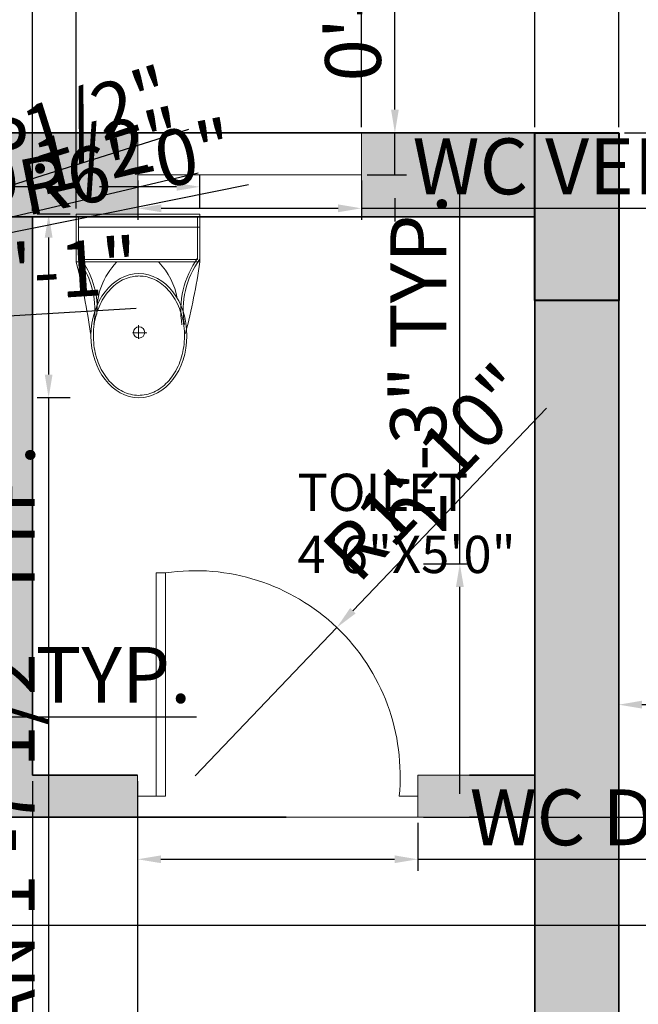
# Model space of a CAD drawing. Units: inches. Extents: x 2656 to 9931, y 1941 to 3068.
# Tile 23 of 46: x 2934 to 3000, y 2530 to 2636. Entities that reach past the tile are written whole.
import ezdxf

# ---------------------------------------------------------------- set-up
doc = ezdxf.new("R2010")
doc.units = ezdxf.units.IN
for name, color, linetype, lineweight in [('A-ANNO-DIMS', 2, 'Continuous', 18), ('A-AREA-IDEN', 7, 'Continuous', 18), ('A-COLS', 7, 'Continuous', 40), ('A-COLS-PATT', 146, 'Continuous', 13), ('A-DOOR', 3, 'Continuous', 18), ('A-FLOR-FIXT', 9, 'Continuous', 18), ('A-GLAZ', 4, 'Continuous', 18), ('A-WALL', 7, 'Continuous', 35), ('A-WALL-PATT', 251, 'Continuous', 13)]:
    doc.layers.add(name, color=color, linetype=linetype, lineweight=lineweight)
doc.styles.get("Standard").update_dxf_attribs({"font": 'arial.ttf'})
doc.dimstyles.new('ISO-25', dxfattribs={"dimtxt": 6, "dimasz": 2.5, "dimexe": 1.25, "dimexo": 0.625, "dimtad": 1, "dimdec": 0, "dimlunit": 3, "dimtxsty": 'Standard', "dimcen": 2.5, "dimadec": 0, "dimazin": 0, "dimtfac": 1, "dimtdec": 0, "dimtmove": 0, "dimatfit": 3, "dimfxl": 1, "dimarcsym": 0})

# ---------------------------------------------------------------- blocks, each defined once
blk = doc.blocks.new('*D3')
at = {"layer": 'A-ANNO-DIMS', "color": 0, "lineweight": -2, "transparency": 16777216}
for p, q in [((2998.16, 2562.82), (2998.16, 2563.44)), ((3028.16, 2562.82), (3028.16, 2563.44)), ((3000.66, 2562.19), (3025.66, 2562.19))]:
    blk.add_line(p, q, dxfattribs=at)
at = {"layer": 'A-ANNO-DIMS', "color": 0, "transparency": 16777216}
for points in [[(3000.66, 2562.61), (3000.66, 2561.77), (2998.16, 2562.19)], [(3025.66, 2562.61), (3025.66, 2561.77), (3028.16, 2562.19)]]:
    blk.add_solid(points, dxfattribs=at)
at = {"layer": 'Defpoints', "color": 0, "transparency": 16777216}
for p in [(2998.16, 2562.19), (3028.16, 2562.19), (3028.16, 2562.19)]:
    blk.add_point(p, dxfattribs=at)
at = {"layer": 'A-ANNO-DIMS', "color": 0, "transparency": 16777216, "insert": (3013.16, 2565.88), "char_height": 6, "attachment_point": 5}
blk.add_mtext('2\'6"', dxfattribs=at)
blk = doc.blocks.new('A$C31115884')
for p, q in [((283.1, 497.7), (223.4, 497.7)), ((257.5, 466.4), (257.5, 523.2)), ((0, 200), (0, 0)), ((520, 200), (0, 200)), ((10, 190), (10, 10)), ((510, 190), (10, 190)), ((510, 10), (510, 190)), ((520, 0), (520, 200)), ((510, 54.5), (0, 54.5)), ((10, 10), (510, 10)), ((0, 0), (520, 0))]:
    blk.add_line(p, q)
blk.add_circle((255.6, 496.4), 23.6)
for centre, radius, start, end in [((2777.7, -204.6), 2807, 165.4549, 171.7133), ((3237, 905), 2807, 188.2867, 194.5451), ((-294.5, 403.3), 364.7, 324.2091, 9.3499), ((-294.5, 403.3), 374.7, 324.2091, 9.3499), ((805.8, 403.3), 364.7, 170.6501, 215.7909), ((139.5, 406.2), 293.5, 315.8436, 2.6563), ((805.8, 403.3), 374.7, 179.2036, 215.7909), ((383.6, 406.2), 293.5, 190.2774, 224.1564)]:
    blk.add_arc(centre, radius, start, end)
blk.add_ellipse((256.2, 509.9), major_axis=(0, -260.7), ratio=0.772727)
blk.add_open_spline([(256.2, 259.2), (263.1, 259.2), (270, 259.7), (287.8, 262.3), (298.7, 265.1), (319.9, 273.1), (330.2, 278.4), (350.1, 291.1), (359.7, 298.7), (377.7, 315.9), (386.2, 325.5), (401.7, 346.6), (408.8, 358.1), (421.3, 382.5), (426.8, 395.5), (435.9, 422.4), (439.5, 436.4), (444.8, 465.1), (446.5, 479.7), (447.9, 509.2), (447.6, 524), (445, 553.3), (442.7, 567.8), (436.3, 596), (432.1, 609.7), (421.9, 636), (416, 648.6), (402.5, 672.1), (395, 683), (378.6, 703), (369.8, 712.1), (351.1, 728), (341.3, 734.8), (320.9, 746.2), (310.4, 750.7), (288.9, 757.3), (278, 759.4), (256, 761), (245, 760.6), (223.1, 757.2), (212.3, 754.3), (191.1, 746.1), (180.8, 740.7), (160.9, 727.8), (151.4, 720.1), (133.5, 702.7), (125.1, 693), (109.6, 671.7), (102.6, 660.2), (90.2, 635.7), (84.9, 622.7), (76, 595.6), (72.4, 581.6), (67.2, 552.9), (65.6, 538.2), (64.4, 508.8), (64.8, 494), (67.5, 464.7), (69.9, 450.2), (76.6, 422), (80.8, 408.3), (91.1, 382.2), (97.2, 369.7), (110.8, 346.3), (118.4, 335.4), (134.8, 315.6), (143.7, 306.7), (162.4, 290.9), (172.3, 284.2), (192.8, 273), (203.3, 268.6), (224.8, 262.2), (235.8, 260.2), (249.9, 259.3), (253, 259.2), (256.2, 259.2)], degree=3, knots=[0, 0, 0, 0, 0.110105, 0.110105, 0.285049, 0.285049, 0.459994, 0.459994, 0.634938, 0.634938, 0.809882, 0.809882, 0.984827, 0.984827, 1.159771, 1.159771, 1.334715, 1.334715, 1.50966, 1.50966, 1.684604, 1.684604, 1.859549, 1.859549, 2.034493, 2.034493, 2.209437, 2.209437, 2.384382, 2.384382, 2.559326, 2.559326, 2.73427, 2.73427, 2.909215, 2.909215, 3.084159, 3.084159, 3.259103, 3.259103, 3.434048, 3.434048, 3.608992, 3.608992, 3.783936, 3.783936, 3.958881, 3.958881, 4.133825, 4.133825, 4.30877, 4.30877, 4.483714, 4.483714, 4.658658, 4.658658, 4.833603, 4.833603, 5.008547, 5.008547, 5.183491, 5.183491, 5.358436, 5.358436, 5.53338, 5.53338, 5.708324, 5.708324, 5.883269, 5.883269, 6.058213, 6.058213, 6.233158, 6.233158, 6.283185, 6.283185, 6.283185, 6.283185])
blk = doc.blocks.new('DOOR-WC-FRONT')
for p, q in [((1.97, 2.25), (1.97, 26.25)), ((1.97, 26.25), (2.97, 26.25)), ((2.97, 26.25), (2.97, 2.25)), ((-0.03, 2.25), (1.97, 2.25)), ((2.97, 2.25), (1.97, 2.25)), ((30.07, 2.25), (28.07, 2.25)), ((-0.03, 0), (30.07, 0))]:
    blk.add_line(p, q)
blk.add_arc((6.14, 4.44), 22.04, 354.3038, 98.2673)
blk = doc.blocks.new('WIN-VENT-24IN-B')
for p, q in [((24.01, 0), (24.01, 4.5)), ((0.01, 0), (0.01, 0)), ((0.01, 0), (24.01, 0))]:
    blk.add_line(p, q)
blk = doc.blocks.new('*D29')
at = {"layer": 'A-ANNO-DIMS', "color": 0, "lineweight": -2, "transparency": 16777216}
for p, q in [((2939.24, 2614.86), (2935.66, 2614.86)), ((2936.91, 2612.36), (2936.91, 2597.65)), ((2939.24, 2595.15), (2935.66, 2595.15)), ((2936.91, 2595.15), (2936.91, 2504.75))]:
    blk.add_line(p, q, dxfattribs=at)
at = {"layer": 'A-ANNO-DIMS', "color": 0, "transparency": 16777216}
for points in [[(2936.49, 2612.36), (2937.33, 2612.36), (2936.91, 2614.86)], [(2936.49, 2597.65), (2937.33, 2597.65), (2936.91, 2595.15)]]:
    blk.add_solid(points, dxfattribs=at)
at = {"layer": 'Defpoints', "color": 0, "transparency": 16777216}
for p in [(2939.87, 2614.86), (2936.91, 2595.15), (2939.87, 2595.15)]:
    blk.add_point(p, dxfattribs=at)
at = {"layer": 'A-ANNO-DIMS', "color": 0, "transparency": 16777216, "insert": (2933.18, 2548.7), "char_height": 6, "attachment_point": 5, "rotation": 90}
blk.add_mtext('WC PAN 1\'-7 1/2" TYP.', dxfattribs=at)
blk = doc.blocks.new('*D30')
at = {"layer": 'A-ANNO-DIMS', "color": 0, "lineweight": -2, "transparency": 16777216}
for p, q in [((2939.87, 2615.48), (2939.87, 2619.06)), ((2953.16, 2615.48), (2953.16, 2619.06)), ((2939.87, 2617.81), (2886.13, 2617.81)), ((2950.66, 2617.81), (2942.37, 2617.81))]:
    blk.add_line(p, q, dxfattribs=at)
at = {"layer": 'A-ANNO-DIMS', "color": 0, "transparency": 16777216}
for points in [[(2942.37, 2618.23), (2942.37, 2617.39), (2939.87, 2617.81)], [(2950.66, 2618.23), (2950.66, 2617.39), (2953.16, 2617.81)]]:
    blk.add_solid(points, dxfattribs=at)
at = {"layer": 'Defpoints', "color": 0, "transparency": 16777216}
for p in [(2939.87, 2617.81), (2939.87, 2614.86), (2953.16, 2614.86)]:
    blk.add_point(p, dxfattribs=at)
at = {"layer": 'A-ANNO-DIMS', "color": 0, "transparency": 16777216, "insert": (2911.75, 2621.54), "char_height": 6, "attachment_point": 5}
blk.add_mtext('1\'-1 1/2" TYP.', dxfattribs=at)
blk = doc.blocks.new('*D34')
at = {"layer": 'A-ANNO-DIMS', "color": 0, "lineweight": -2, "transparency": 16777216}
for p, q in [((2872.16, 2564.71), (2872.16, 2559.64)), ((2898.41, 2564.71), (2898.41, 2559.64)), ((2874.66, 2560.89), (2895.91, 2560.89)), ((2898.41, 2560.89), (2952.81, 2560.89))]:
    blk.add_line(p, q, dxfattribs=at)
at = {"layer": 'A-ANNO-DIMS', "color": 0, "transparency": 16777216}
for points in [[(2874.66, 2561.3), (2874.66, 2560.47), (2872.16, 2560.89)], [(2895.91, 2561.3), (2895.91, 2560.47), (2898.41, 2560.89)]]:
    blk.add_solid(points, dxfattribs=at)
at = {"layer": 'Defpoints', "color": 0, "transparency": 16777216}
for p in [(2872.16, 2565.34), (2898.41, 2565.34), (2898.41, 2560.89)]:
    blk.add_point(p, dxfattribs=at)
at = {"layer": 'A-ANNO-DIMS', "color": 0, "transparency": 16777216, "insert": (2926.86, 2564.61), "char_height": 6, "attachment_point": 5}
blk.add_mtext('2\'-2 1/2" TYP.', dxfattribs=at)
blk = doc.blocks.new('*D35')
at = {"layer": 'A-ANNO-DIMS', "color": 0, "lineweight": -2, "transparency": 16777216}
for p, q in [((2946.47, 2549.48), (2946.47, 2544.33)), ((2976.57, 2549.48), (2976.57, 2544.33)), ((2948.97, 2545.58), (2974.07, 2545.58)), ((2976.57, 2545.58), (3060.91, 2545.58))]:
    blk.add_line(p, q, dxfattribs=at)
at = {"layer": 'A-ANNO-DIMS', "color": 0, "transparency": 16777216}
for points in [[(2948.97, 2546), (2948.97, 2545.17), (2946.47, 2545.58)], [(2974.07, 2546), (2974.07, 2545.17), (2976.57, 2545.58)]]:
    blk.add_solid(points, dxfattribs=at)
at = {"layer": 'Defpoints', "color": 0, "transparency": 16777216}
for p in [(2946.47, 2550.1), (2976.57, 2550.1), (2976.57, 2545.58)]:
    blk.add_point(p, dxfattribs=at)
at = {"layer": 'A-ANNO-DIMS', "color": 0, "transparency": 16777216, "insert": (3019.99, 2549.31), "char_height": 6, "attachment_point": 5}
blk.add_mtext('WC DOOR 2\'-6" TYP.', dxfattribs=at)
blk = doc.blocks.new('*D36')
at = {"layer": 'A-ANNO-DIMS', "color": 0, "lineweight": -2, "transparency": 16777216}
for p, q in [((2981.09, 2577.33), (2981.09, 2617.75)), ((2977.2, 2577.33), (2982.34, 2577.33)), ((2981.09, 2552.6), (2981.09, 2574.83)), ((2977.2, 2550.1), (2982.34, 2550.1))]:
    blk.add_line(p, q, dxfattribs=at)
at = {"layer": 'A-ANNO-DIMS', "color": 0, "transparency": 16777216}
for points in [[(2980.67, 2574.83), (2981.51, 2574.83), (2981.09, 2577.33)], [(2980.67, 2552.6), (2981.51, 2552.6), (2981.09, 2550.1)]]:
    blk.add_solid(points, dxfattribs=at)
at = {"layer": 'Defpoints', "color": 0, "transparency": 16777216}
for p in [(2976.57, 2577.33), (2981.09, 2577.33), (2976.57, 2550.1)]:
    blk.add_point(p, dxfattribs=at)
at = {"layer": 'A-ANNO-DIMS', "color": 0, "transparency": 16777216, "insert": (2977.4, 2598.79), "char_height": 6, "attachment_point": 5, "rotation": 90}
blk.add_mtext('2\'-3" TYP.', dxfattribs=at)
blk = doc.blocks.new('*D45')
at = {"layer": 'A-ANNO-DIMS', "color": 0, "lineweight": -2, "transparency": 16777216}
for p, q in [((2946.51, 2618.48), (2946.51, 2614.25)), ((2970.51, 2618.48), (2970.51, 2614.25)), ((2949.01, 2615.5), (2968.01, 2615.5)), ((2970.51, 2615.5), (3052.06, 2615.5))]:
    blk.add_line(p, q, dxfattribs=at)
at = {"layer": 'A-ANNO-DIMS', "color": 0, "transparency": 16777216}
for points in [[(2949.01, 2615.92), (2949.01, 2615.08), (2946.51, 2615.5)], [(2968.01, 2615.92), (2968.01, 2615.08), (2970.51, 2615.5)]]:
    blk.add_solid(points, dxfattribs=at)
at = {"layer": 'Defpoints', "color": 0, "transparency": 16777216}
for p in [(2946.51, 2619.1), (2970.51, 2619.1), (2970.51, 2615.5)]:
    blk.add_point(p, dxfattribs=at)
at = {"layer": 'A-ANNO-DIMS', "color": 0, "transparency": 16777216, "insert": (3012.54, 2619.23), "char_height": 6, "attachment_point": 5}
blk.add_mtext('WC VENT 2\'-0" TYP.', dxfattribs=at)
blk = doc.blocks.new('*D46')
at = {"layer": 'A-ANNO-DIMS', "color": 0, "lineweight": -2, "transparency": 16777216}
for p, q in [((2974.11, 2626.1), (2974.11, 2680.4)), ((2971.14, 2623.6), (2975.36, 2623.6)), ((2974.11, 2619.1), (2974.11, 2623.6)), ((2971.14, 2619.1), (2975.36, 2619.1)), ((2974.11, 2616.6), (2974.11, 2614.1))]:
    blk.add_line(p, q, dxfattribs=at)
at = {"layer": 'A-ANNO-DIMS', "color": 0, "transparency": 16777216}
for points in [[(2973.7, 2626.1), (2974.53, 2626.1), (2974.11, 2623.6)], [(2973.7, 2616.6), (2974.53, 2616.6), (2974.11, 2619.1)]]:
    blk.add_solid(points, dxfattribs=at)
at = {"layer": 'Defpoints', "color": 0, "transparency": 16777216}
for p in [(2970.51, 2623.6), (2974.11, 2623.6), (2970.51, 2619.1)]:
    blk.add_point(p, dxfattribs=at)
at = {"layer": 'A-ANNO-DIMS', "color": 0, "transparency": 16777216, "insert": (2970.39, 2654.5), "char_height": 6, "attachment_point": 5, "rotation": 90}
blk.add_mtext('0\'-4 1/2" TYP.', dxfattribs=at)
blk = doc.blocks.new('*D99')
at = {"layer": 'A-ANNO-DIMS', "color": 0, "lineweight": -2, "transparency": 16777216}
for p, q in [((2970.51, 2624.23), (2970.51, 2674.45)), ((2989.16, 2624.23), (2989.16, 2674.45)), ((2973.01, 2673.2), (2986.66, 2673.2)), ((2989.16, 2673.2), (3022.27, 2673.2))]:
    blk.add_line(p, q, dxfattribs=at)
at = {"layer": 'A-ANNO-DIMS', "color": 0, "transparency": 16777216}
for points in [[(2973.01, 2673.62), (2973.01, 2672.78), (2970.51, 2673.2)], [(2986.66, 2673.62), (2986.66, 2672.78), (2989.16, 2673.2)]]:
    blk.add_solid(points, dxfattribs=at)
at = {"layer": 'Defpoints', "color": 0, "transparency": 16777216}
for p in [(2989.16, 2673.2), (2970.51, 2623.6), (2989.16, 2623.6)]:
    blk.add_point(p, dxfattribs=at)
at = {"layer": 'A-ANNO-DIMS', "color": 0, "transparency": 16777216, "insert": (3006.97, 2676.93), "char_height": 6, "attachment_point": 5}
blk.add_mtext('1\'-6 1/2"', dxfattribs=at)
blk = doc.blocks.new('*D101')
at = {"layer": 'A-ANNO-DIMS', "color": 0, "lineweight": -2, "transparency": 16777216}
for p, q in [((2935.16, 2553.98), (2935.16, 2009.27)), ((2946.47, 2553.98), (2946.47, 2009.27)), ((2937.66, 2010.52), (2943.97, 2010.52)), ((2946.47, 2010.52), (2984.81, 2010.52))]:
    blk.add_line(p, q, dxfattribs=at)
at = {"layer": 'A-ANNO-DIMS', "color": 0, "transparency": 16777216}
for points in [[(2937.66, 2010.94), (2937.66, 2010.11), (2935.16, 2010.52)], [(2943.97, 2010.94), (2943.97, 2010.11), (2946.47, 2010.52)]]:
    blk.add_solid(points, dxfattribs=at)
at = {"layer": 'Defpoints', "color": 0, "transparency": 16777216}
for p in [(2935.16, 2554.6), (2946.47, 2554.6), (2946.47, 2010.52)]:
    blk.add_point(p, dxfattribs=at)
at = {"layer": 'A-ANNO-DIMS', "color": 0, "transparency": 16777216, "insert": (2966.89, 2014.25), "char_height": 6, "attachment_point": 5}
blk.add_mtext('0\'-11 1/2"', dxfattribs=at)
blk = doc.blocks.new('*D102')
at = {"layer": 'A-ANNO-DIMS', "color": 0, "lineweight": -2, "transparency": 16777216}
for p, q in [((2998.16, 2604.98), (2998.16, 2009.27)), ((2872.16, 2564.71), (2872.16, 2009.27)), ((2874.66, 2010.52), (2995.66, 2010.52))]:
    blk.add_line(p, q, dxfattribs=at)
at = {"layer": 'A-ANNO-DIMS', "color": 0, "transparency": 16777216}
for points in [[(2874.66, 2010.94), (2874.66, 2010.11), (2872.16, 2010.52)], [(2995.66, 2010.94), (2995.66, 2010.11), (2998.16, 2010.52)]]:
    blk.add_solid(points, dxfattribs=at)
at = {"layer": 'Defpoints', "color": 0, "transparency": 16777216}
for p in [(2998.16, 2605.6), (2872.16, 2565.34), (2998.16, 2010.52)]:
    blk.add_point(p, dxfattribs=at)
at = {"layer": 'A-ANNO-DIMS', "color": 0, "transparency": 16777216, "insert": (2935.16, 2014.21), "char_height": 6, "attachment_point": 5}
blk.add_mtext('10\'-6"', dxfattribs=at)
blk = doc.blocks.new('*D103')
at = {"layer": 'A-ANNO-DIMS', "color": 0, "lineweight": -2, "transparency": 16777216}
for p, q in [((2998.78, 2623.6), (3061.01, 2623.6)), ((3059.76, 2552.6), (3059.76, 2621.1)), ((2989.78, 2550.1), (3061.01, 2550.1))]:
    blk.add_line(p, q, dxfattribs=at)
at = {"layer": 'A-ANNO-DIMS', "color": 0, "transparency": 16777216}
for points in [[(3059.34, 2621.1), (3060.17, 2621.1), (3059.76, 2623.6)], [(3059.34, 2552.6), (3060.17, 2552.6), (3059.76, 2550.1)]]:
    blk.add_solid(points, dxfattribs=at)
at = {"layer": 'Defpoints', "color": 0, "transparency": 16777216}
for p in [(2998.16, 2623.6), (3059.76, 2623.6), (2989.16, 2550.1)]:
    blk.add_point(p, dxfattribs=at)
at = {"layer": 'A-ANNO-DIMS', "color": 0, "transparency": 16777216, "insert": (3056.03, 2586.85), "char_height": 6, "attachment_point": 5, "rotation": 90}
blk.add_mtext('6\'-1 1/2"', dxfattribs=at)
blk = doc.blocks.new('*D130')
at = {"layer": 'A-ANNO-DIMS', "color": 0, "lineweight": -2, "transparency": 16777216}
for p, q in [((2877.28, 2538.52), (3061.01, 2538.52)), ((3059.76, 2536.02), (3059.76, 2525.32)), ((2902.17, 2522.82), (3061.01, 2522.82)), ((3059.76, 2522.82), (3059.76, 2489.7))]:
    blk.add_line(p, q, dxfattribs=at)
at = {"layer": 'A-ANNO-DIMS', "color": 0, "transparency": 16777216}
for points in [[(3059.34, 2536.02), (3060.17, 2536.02), (3059.76, 2538.52)], [(3059.34, 2525.32), (3060.17, 2525.32), (3059.76, 2522.82)]]:
    blk.add_solid(points, dxfattribs=at)
at = {"layer": 'Defpoints', "color": 0, "transparency": 16777216}
for p in [(2876.66, 2538.52), (2901.54, 2522.82), (3059.76, 2522.82)]:
    blk.add_point(p, dxfattribs=at)
at = {"layer": 'A-ANNO-DIMS', "color": 0, "transparency": 16777216, "insert": (3056.03, 2505.01), "char_height": 6, "attachment_point": 5, "rotation": 90}
blk.add_mtext('1\'-3 1/2"', dxfattribs=at)
blk = doc.blocks.new('*D174')
at = {"layer": 'A-ANNO-DIMS', "color": 0, "lineweight": -2, "transparency": 16777216}
for p, q in [((2743.16, 2624.23), (2743.16, 2674.45)), ((2998.16, 2624.23), (2998.16, 2674.45)), ((2745.66, 2673.2), (2995.66, 2673.2))]:
    blk.add_line(p, q, dxfattribs=at)
at = {"layer": 'A-ANNO-DIMS', "color": 0, "transparency": 16777216}
for points in [[(2745.66, 2673.62), (2745.66, 2672.78), (2743.16, 2673.2)], [(2995.66, 2673.62), (2995.66, 2672.78), (2998.16, 2673.2)]]:
    blk.add_solid(points, dxfattribs=at)
at = {"layer": 'Defpoints', "color": 0, "transparency": 16777216}
for p in [(2998.16, 2673.2), (2743.16, 2623.6), (2998.16, 2623.6)]:
    blk.add_point(p, dxfattribs=at)
at = {"layer": 'A-ANNO-DIMS', "color": 0, "transparency": 16777216, "insert": (2870.66, 2676.89), "char_height": 6, "attachment_point": 5}
blk.add_mtext('21\'-3"', dxfattribs=at)
blk = doc.blocks.new('*D177')
at = {"layer": 'A-ANNO-DIMS', "color": 0, "lineweight": -2, "transparency": 16777216}
for p, q in [((2935.16, 2615.23), (2935.16, 2674.45)), ((2939.87, 2615.48), (2939.87, 2674.45)), ((2932.66, 2673.2), (2930.16, 2673.2)), ((2935.16, 2673.2), (2939.87, 2673.2)), ((2942.37, 2673.2), (2976.05, 2673.2))]:
    blk.add_line(p, q, dxfattribs=at)
at = {"layer": 'A-ANNO-DIMS', "color": 0, "transparency": 16777216}
for points in [[(2932.66, 2673.62), (2932.66, 2672.78), (2935.16, 2673.2)], [(2942.37, 2673.62), (2942.37, 2672.78), (2939.87, 2673.2)]]:
    blk.add_solid(points, dxfattribs=at)
at = {"layer": 'Defpoints', "color": 0, "transparency": 16777216}
for p in [(2939.87, 2673.2), (2935.16, 2614.6), (2939.87, 2614.86)]:
    blk.add_point(p, dxfattribs=at)
at = {"layer": 'A-ANNO-DIMS', "color": 0, "transparency": 16777216, "insert": (2960.46, 2676.93), "char_height": 6, "attachment_point": 5}
blk.add_mtext('0\'-4 1/2"', dxfattribs=at)
blk = doc.blocks.new('*D187')
at = {"layer": 'A-ANNO-DIMS', "color": 0, "lineweight": -2, "transparency": 16777216}
for p, q in [((2990.41, 2594.03), (2969.6, 2572.28)), ((2952.64, 2554.54), (2967.87, 2570.47))]:
    blk.add_line(p, q, dxfattribs=at)
at = {"layer": 'A-ANNO-DIMS', "color": 0, "transparency": 16777216}
blk.add_solid([(2969.3, 2572.56), (2969.9, 2571.99), (2967.87, 2570.47)], dxfattribs=at)
at = {"layer": 'Defpoints', "color": 0, "transparency": 16777216}
for p in [(2967.87, 2570.47), (2952.64, 2554.54)]:
    blk.add_point(p, dxfattribs=at)
at = {"layer": 'A-ANNO-DIMS', "color": 0, "transparency": 16777216, "insert": (2978.2, 2586.61), "char_height": 6, "attachment_point": 5, "rotation": 46.2844}
blk.add_mtext('R1\'-10"', dxfattribs=at)
blk = doc.blocks.new('*D189')
at = {"layer": 'A-ANNO-DIMS', "color": 0, "lineweight": -2, "transparency": 16777216}
for p, q in [((2958.39, 2618.02), (2900.95, 2606.42)), ((2828.14, 2591.72), (2898.5, 2605.92))]:
    blk.add_line(p, q, dxfattribs=at)
at = {"layer": 'A-ANNO-DIMS', "color": 0, "transparency": 16777216}
blk.add_solid([(2900.86, 2606.83), (2901.03, 2606.01), (2898.5, 2605.92)], dxfattribs=at)
at = {"layer": 'Defpoints', "color": 0, "transparency": 16777216}
for p in [(2898.5, 2605.92), (2828.14, 2591.72)]:
    blk.add_point(p, dxfattribs=at)
at = {"layer": 'A-ANNO-DIMS', "color": 0, "transparency": 16777216, "insert": (2939.98, 2618.06), "char_height": 6, "attachment_point": 5, "rotation": 11.4157}
blk.add_mtext('4X R6\'-0"', dxfattribs=at)
blk = doc.blocks.new('*D190')
at = {"layer": 'A-ANNO-DIMS', "color": 0, "lineweight": -2, "transparency": 16777216}
for p, q in [((2951.95, 2623.98), (2901.83, 2608.18)), ((2890.31, 2604.54), (2899.44, 2607.42))]:
    blk.add_line(p, q, dxfattribs=at)
at = {"layer": 'A-ANNO-DIMS', "color": 0, "transparency": 16777216}
blk.add_solid([(2901.7, 2608.57), (2901.95, 2607.78), (2899.44, 2607.42)], dxfattribs=at)
at = {"layer": 'Defpoints', "color": 0, "transparency": 16777216}
for p in [(2899.44, 2607.42), (2890.31, 2604.54)]:
    blk.add_point(p, dxfattribs=at)
at = {"layer": 'A-ANNO-DIMS', "color": 0, "transparency": 16777216, "insert": (2926.96, 2620.01), "char_height": 6, "attachment_point": 5, "rotation": 17.4987}
blk.add_mtext('4X R0\'-9 1/2"', dxfattribs=at)
blk = doc.blocks.new('*D191')
at = {"layer": 'A-ANNO-DIMS', "color": 0, "lineweight": -2, "transparency": 16777216}
for p, q in [((2952.98, 2619.27), (2901.82, 2607.25)), ((2890.31, 2604.54), (2899.39, 2606.68))]:
    blk.add_line(p, q, dxfattribs=at)
at = {"layer": 'A-ANNO-DIMS', "color": 0, "transparency": 16777216}
blk.add_solid([(2901.72, 2607.65), (2901.91, 2606.84), (2899.39, 2606.68)], dxfattribs=at)
at = {"layer": 'Defpoints', "color": 0, "transparency": 16777216}
for p in [(2899.39, 2606.68), (2890.31, 2604.54)]:
    blk.add_point(p, dxfattribs=at)
at = {"layer": 'A-ANNO-DIMS', "color": 0, "transparency": 16777216, "insert": (2927.76, 2617.17), "char_height": 6, "attachment_point": 5, "rotation": 13.2221}
blk.add_mtext('4X R0\'-9 1/2"', dxfattribs=at)
blk = doc.blocks.new('*D193')
at = {"layer": 'A-ANNO-DIMS', "color": 0, "lineweight": -2, "transparency": 16777216}
for p, q in [((2946.3, 2604.75), (2907.47, 2602.35)), ((2901.28, 2601.97), (2898.78, 2601.82)), ((2903.77, 2602.12), (2904.98, 2602.2))]:
    blk.add_line(p, q, dxfattribs=at)
at = {"layer": 'A-ANNO-DIMS', "color": 0, "transparency": 16777216}
for points in [[(2907.45, 2602.77), (2907.5, 2601.94), (2904.98, 2602.2)], [(2901.25, 2602.39), (2901.3, 2601.55), (2903.77, 2602.12)]]:
    blk.add_solid(points, dxfattribs=at)
at = {"layer": 'Defpoints', "color": 0, "transparency": 16777216}
for p in [(2903.77, 2602.12), (2904.98, 2602.2)]:
    blk.add_point(p, dxfattribs=at)
at = {"layer": 'A-ANNO-DIMS', "color": 0, "transparency": 16777216, "insert": (2927.9, 2607.48), "char_height": 6, "attachment_point": 5, "rotation": 3.5337}
blk.add_mtext('2X ∅0\'-1"', dxfattribs=at)

msp = doc.modelspace()

# ---------------------------------------------------------------- hatches: boundary and pattern name
at = {"layer": 'A-COLS-PATT'}
h = msp.add_hatch(color=256, dxfattribs=at)
h.dxf.hatch_style = 1
h.paths.add_polyline_path([(2752.16, 2623.6), (2743.16, 2623.6), (2743.16, 2605.6), (2752.16, 2605.6)])
h.paths.add_polyline_path([(2876.66, 2623.6), (2858.66, 2623.6), (2858.66, 2614.6), (2876.66, 2614.6)])
h.paths.add_polyline_path([(2998.16, 2623.6), (2989.16, 2623.6), (2989.16, 2614.6), (2989.16, 2605.6), (2998.16, 2605.6)])
h.paths.add_polyline_path([(2998.16, 2444.1), (2989.16, 2444.1), (2989.16, 2426.1), (2998.16, 2426.1)])
h.paths.add_polyline_path([(2876.66, 2444.1), (2867.66, 2444.1), (2867.66, 2426.1), (2876.66, 2426.1)])
h.paths.add_polyline_path([(2752.16, 2444.1), (2743.16, 2444.1), (2743.16, 2426.1), (2752.16, 2426.1)])
h.paths.add_polyline_path([(2752.16, 2300.1), (2743.16, 2300.1), (2743.16, 2282.1), (2752.16, 2282.1)])
h.paths.add_polyline_path([(2876.66, 2300.1), (2867.66, 2300.1), (2867.66, 2282.1), (2876.66, 2282.1)])
h.paths.add_polyline_path([(2998.16, 2300.1), (2989.16, 2300.1), (2989.16, 2282.1), (2998.16, 2282.1)])
h.paths.add_polyline_path([(2998.16, 2184.6), (2989.16, 2184.6), (2989.16, 2166.6), (2998.16, 2166.6)])
h.paths.add_polyline_path([(2876.66, 2175.6), (2858.66, 2175.6), (2858.66, 2166.6), (2876.66, 2166.6)])
h.paths.add_polyline_path([(2752.16, 2184.6), (2743.16, 2184.6), (2743.16, 2166.6), (2752.16, 2166.6)])
at = {"layer": 'A-WALL-PATT'}
h = msp.add_hatch(color=256, dxfattribs=at)
h.dxf.hatch_style = 1
h.paths.add_polyline_path([(2858.66, 2623.6), (2752.16, 2623.6), (2752.16, 2614.6), (2858.66, 2614.6)])
h.paths.add_polyline_path([(2893.09, 2623.6), (2876.66, 2623.6), (2876.66, 2614.6), (2893.09, 2614.6), (2893.09, 2619.1)])
h.paths.add_polyline_path([(2946.51, 2623.6), (2917.09, 2623.6), (2917.09, 2614.6), (2946.51, 2614.6), (2946.51, 2619.1)])
h.paths.add_polyline_path([(2989.16, 2623.6), (2970.51, 2623.6), (2970.51, 2614.6), (2989.16, 2614.6)])
h.paths.add_polyline_path([(2998.16, 2605.6), (2989.16, 2605.6), (2989.16, 2523.88), (2998.16, 2523.88)])
h.paths.add_polyline_path([(2935.16, 2614.6), (2930.66, 2614.6), (2930.66, 2554.6), (2876.66, 2554.6), (2876.66, 2565.34), (2872.16, 2565.34), (2872.16, 2444.1), (2876.66, 2444.1), (2876.66, 2550.1), (2946.47, 2550.1), (2946.47, 2554.6), (2935.16, 2554.6)])
h.paths.add_polyline_path([(2989.16, 2554.6), (2982.11, 2554.6), (2976.57, 2554.6), (2976.57, 2550.1), (2982.11, 2550.1), (2989.16, 2550.1)])
h.paths.add_polyline_path([(2876.66, 2614.6), (2872.16, 2614.6), (2872.16, 2595), (2876.66, 2595)], flags=0)
h.paths.add_polyline_path([(2752.16, 2605.6), (2743.16, 2605.6), (2743.16, 2544.03), (2752.16, 2544.03)])
h.paths.add_polyline_path([(2752.16, 2426.1), (2743.16, 2426.1), (2743.16, 2300.1), (2752.16, 2300.1)])
h.paths.add_polyline_path([(2821.13, 2430.6), (2752.16, 2430.6), (2752.16, 2426.1), (2821.13, 2426.1)])
h.paths.add_polyline_path([(2867.66, 2430.6), (2862.88, 2430.6), (2862.88, 2426.1), (2867.66, 2426.1)])
h.paths.add_polyline_path([(2752.16, 2484.03), (2747.66, 2484.03), (2743.16, 2484.03), (2743.16, 2444.1), (2752.16, 2444.1)])
h.paths.add_polyline_path([(2998.16, 2426.1), (2989.16, 2426.1), (2989.16, 2390.1), (2872.16, 2390.1), (2872.16, 2385.6), (2876.66, 2385.6), (2989.16, 2385.6), (2989.16, 2365.04), (2998.16, 2365.04)])
h.paths.add_polyline_path([(2998.16, 2463.88), (2993.66, 2463.88), (2989.16, 2463.88), (2989.16, 2444.1), (2998.16, 2444.1)])
h.paths.add_polyline_path([(2998.16, 2319.88), (2989.16, 2319.88), (2989.16, 2300.1), (2998.16, 2300.1)])
h.paths.add_polyline_path([(2998.16, 2282.1), (2989.16, 2282.1), (2989.16, 2253.6), (2982.06, 2253.6), (2982.06, 2249.1), (2989.16, 2249.1), (2998.16, 2249.1)])
h.paths.add_polyline_path([(2931.54, 2253.6), (2923.8, 2253.6), (2923.8, 2249.1), (2931.54, 2249.1)])
h.paths.add_polyline_path([(2876.66, 2282.1), (2872.16, 2282.1), (2872.16, 2184.6), (2872.16, 2175.6), (2876.66, 2175.6), (2876.66, 2249.1), (2888.32, 2249.1), (2888.32, 2251.35), (2888.32, 2253.6), (2876.66, 2253.6)])
h.paths.add_polyline_path([(2858.66, 2175.6), (2841.42, 2175.6), (2841.42, 2166.6), (2858.66, 2166.6)])
h.paths.add_polyline_path([(2785.06, 2171.1), (2785.06, 2175.6), (2752.16, 2175.6), (2752.16, 2166.6), (2785.06, 2166.6)])
h.paths.add_polyline_path([(2752.16, 2282.1), (2743.16, 2282.1), (2743.16, 2184.6), (2752.16, 2184.6)])
h.paths.add_polyline_path([(2809.77, 2300.1), (2752.16, 2300.1), (2752.16, 2295.6), (2809.77, 2295.6)])
h.paths.add_polyline_path([(2867.66, 2300.1), (2851.88, 2300.1), (2851.88, 2295.6), (2867.66, 2295.6)])

# ---------------------------------------------------------------- linework, layer by layer
at = {"layer": 'A-COLS'}
for p, q in [((2989.16, 2614.6), (2989.16, 2623.6)), ((2989.16, 2623.6), (2998.16, 2623.6)), ((2998.16, 2623.6), (2998.16, 2605.6)), ((2989.16, 2605.6), (2989.16, 2614.6)), ((2998.16, 2605.6), (2989.16, 2605.6))]:
    msp.add_line(p, q, dxfattribs=at)
at = {"layer": 'A-DOOR'}
for p, q in [((2946.47, 2554.6), (2946.47, 2550.1)), ((2982.11, 2554.6), (2976.57, 2554.6)), ((2976.57, 2554.6), (2976.57, 2550.1)), ((2976.57, 2550.1), (2982.11, 2550.1))]:
    msp.add_line(p, q, dxfattribs=at)
at = {"layer": 'A-GLAZ'}
for p, q in [((2946.51, 2623.6), (2946.51, 2614.6)), ((2970.51, 2623.6), (2970.51, 2614.6)), ((2946.51, 2614.6), (2946.51, 2619.1))]:
    msp.add_line(p, q, dxfattribs=at)
at = {"layer": 'A-WALL'}
for p, q in [((2743.16, 2623.6), (2998.16, 2623.6)), ((2998.16, 2623.6), (2998.16, 2249.1)), ((2752.16, 2614.6), (2989.16, 2614.6)), ((2935.16, 2614.6), (2935.16, 2554.6)), ((2989.16, 2614.6), (2989.16, 2390.1)), ((2935.16, 2554.6), (2946.47, 2554.6)), ((2982.11, 2554.6), (2989.16, 2554.6)), ((2876.66, 2550.1), (2946.47, 2550.1)), ((2876.66, 2550.1), (2962.42, 2550.1)), ((2982.11, 2550.1), (2989.16, 2550.1))]:
    msp.add_line(p, q, dxfattribs=at)

# ---------------------------------------------------------------- block references
at = {"layer": 'A-DOOR'}
msp.add_blockref('DOOR-WC-FRONT', (2946.5, 2550.1), dxfattribs=at)
at = {"layer": 'A-FLOR-FIXT', "xscale": 0.0255708354650279, "yscale": 0.0255708354650279, "zscale": 0.0255708354650279, "rotation": 180}
msp.add_blockref('A$C31115884', (2953.16, 2614.86), dxfattribs=at)
at = {"layer": 'A-GLAZ'}
msp.add_blockref('WIN-VENT-24IN-B', (2946.5, 2619.1), dxfattribs=at)

# ---------------------------------------------------------------- texts
at = {"layer": 'A-AREA-IDEN', "insert": (2963.64, 2593.66), "char_height": 4, "attachment_point": 1}
msp.add_mtext_dynamic_manual_height_columns('\\PTOILET\\P4\'6"X5\'0"', width=137.4726, gutter_width=12.5, heights=[0], dxfattribs=at)

# ---------------------------------------------------------------- dimensions: what is measured, and where the dimension line sits
at = {"layer": 'A-ANNO-DIMS'}
for base, p1, p2, picture, middle in [((2939.87, 2673.2), (2935.16, 2614.6), (2939.87, 2614.86), '*D177', (2960.46, 2676.93)), ((2989.1573, 2673.2003), (2970.5139, 2623.6003), (2989.1573, 2623.6003), '*D99', (3006.9651, 2676.9276)), ((2998.16, 2673.2), (2743.16, 2623.6), (2998.16, 2623.6), '*D174', (2870.66, 2676.89)), ((2998.16, 2010.52), (2872.16, 2565.34), (2998.16, 2605.6), '*D102', (2935.16, 2014.21)), ((2946.47, 2010.52), (2935.16, 2554.6), (2946.47, 2554.6), '*D101', (2966.89, 2014.25))]:
    dim = msp.add_linear_dim(base=base, p1=p1, p2=p2, dimstyle='ISO-25', override={"dimdec": 1, "dimlfac": 1, "dimrnd": 0, "dimzin": 1, "dimdsep": 46, "dimlunit": 4, "dimfrac": 2}, dxfattribs=at)
    dim.commit()
    dim.dimension.update_dxf_attribs({"geometry": picture, "text_midpoint": middle})
for base, p1, p2, angle, text, picture, middle in [((2974.11, 2623.6), (2970.51, 2619.1), (2970.51, 2623.6), 90, '<> TYP.', '*D46', (2970.39, 2654.5)), ((2939.87, 2617.81), (2953.16, 2614.86), (2939.87, 2614.86), 180, '<> TYP.', '*D30', (2911.75, 2621.54)), ((2981.09, 2577.33), (2976.57, 2550.1), (2976.57, 2577.33), 90, '<> TYP.', '*D36', (2977.4, 2598.79)), ((2936.91, 2595.15), (2939.87, 2614.86), (2939.87, 2595.15), 270, 'WC PAN <> TYP.', '*D29', (2933.18, 2548.7))]:
    dim = msp.add_linear_dim(base=base, p1=p1, p2=p2, angle=angle, text=text, dimstyle='ISO-25', override={"dimdec": 1, "dimlfac": 1, "dimrnd": 0, "dimzin": 1, "dimdsep": 46, "dimlunit": 4, "dimfrac": 2}, dxfattribs=at)
    dim.commit()
    dim.dimension.update_dxf_attribs({"geometry": picture, "text_midpoint": middle})
for base, p1, p2, text, override, picture, middle in [((2970.51, 2615.5), (2946.51, 2619.1), (2970.51, 2619.1), 'WC VENT <> TYP.', {"dimdec": 1, "dimlfac": 1, "dimrnd": 0, "dimzin": 1, "dimdsep": 46, "dimlunit": 4, "dimfrac": 2}, '*D45', (3012.54, 2619.23)), ((2898.40725845, 2560.88740193), (2872.15725845, 2565.33730739), (2898.40725845, 2565.33730739), '<> TYP.', {"dimdec": 1, "dimlfac": 1, "dimrnd": 0, "dimzin": 1, "dimdsep": 46, "dimlunit": 4, "dimfrac": 2}, '*D34', (2926.86036213, 2564.61472116)), ((3028.16, 2562.19), (2998.16, 2562.19), (3028.16, 2562.19), '2\'6"', {"dimclrd": 0, "dimclre": 0, "dimclrt": 0}, '*D3', (3013.16, 2565.88)), ((2976.57, 2545.58), (2946.47, 2550.1), (2976.57, 2550.1), 'WC DOOR <> TYP.', {"dimdec": 1, "dimlfac": 1, "dimrnd": 0, "dimzin": 1, "dimdsep": 46, "dimlunit": 4, "dimfrac": 2}, '*D35', (3019.99, 2549.31))]:
    dim = msp.add_linear_dim(base=base, p1=p1, p2=p2, text=text, dimstyle='ISO-25', override=override, dxfattribs=at)
    dim.commit()
    dim.dimension.update_dxf_attribs({"geometry": picture, "text_midpoint": middle})
for mpoint, picture, middle in [((2899.44, 2607.42), '*D190', (2926.96, 2620.01)), ((2899.39, 2606.68), '*D191', (2927.76, 2617.17))]:
    dim = msp.add_radius_dim(center=(2890.31, 2604.54), mpoint=mpoint, text='4X <>', dimstyle='ISO-25', override={"dimdec": 1, "dimlfac": 1, "dimrnd": 0, "dimzin": 1, "dimdsep": 46, "dimlunit": 4, "dimfrac": 2}, dxfattribs=at)
    dim.commit()
    dim.dimension.update_dxf_attribs({"geometry": picture, "text_midpoint": middle})
dim = msp.add_radius_dim(center=(2828.14, 2591.72), mpoint=(2898.5, 2605.92), text='4X <>', dimstyle='ISO-25', override={"dimdec": 1, "dimlfac": 1, "dimrnd": 0, "dimzin": 1, "dimdsep": 46, "dimlunit": 4, "dimfrac": 2}, dxfattribs=at)
dim.commit()
dim.dimension.update_dxf_attribs({"geometry": '*D189', "text_midpoint": (2940.71, 2614.45), "dimtype": 164})
for base, p1, p2, picture, middle in [((3059.76, 2623.6), (2989.16, 2550.1), (2998.16, 2623.6), '*D103', (3056.03, 2586.85)), ((3059.76, 2522.82), (2876.66, 2538.52), (2901.54, 2522.82), '*D130', (3056.03, 2505.01))]:
    dim = msp.add_linear_dim(base=base, p1=p1, p2=p2, angle=90, dimstyle='ISO-25', override={"dimdec": 1, "dimlfac": 1, "dimrnd": 0, "dimzin": 1, "dimdsep": 46, "dimlunit": 4, "dimfrac": 2}, dxfattribs=at)
    dim.commit()
    dim.dimension.update_dxf_attribs({"geometry": picture, "text_midpoint": middle})
dim = msp.add_diameter_dim_2p(p1=(2903.77, 2602.12), p2=(2904.98, 2602.2), text='2X <>', dimstyle='ISO-25', override={"dimdec": 1, "dimlfac": 1, "dimrnd": 0, "dimzin": 1, "dimdsep": 46, "dimlunit": 4, "dimfrac": 2}, dxfattribs=at)
dim.commit()
dim.dimension.update_dxf_attribs({"geometry": '*D193', "text_midpoint": (2928.14, 2603.63), "dimtype": 163})
dim = msp.add_radius_dim(center=(2952.64, 2554.54), mpoint=(2967.87, 2570.47), dimstyle='ISO-25', override={"dimdec": 1, "dimlfac": 1, "dimrnd": 0, "dimzin": 1, "dimdsep": 46, "dimlunit": 4, "dimfrac": 2}, dxfattribs=at)
dim.commit()
dim.dimension.update_dxf_attribs({"geometry": '*D187', "text_midpoint": (2978.2, 2586.61)})

doc.saveas('drawing.dxf')
